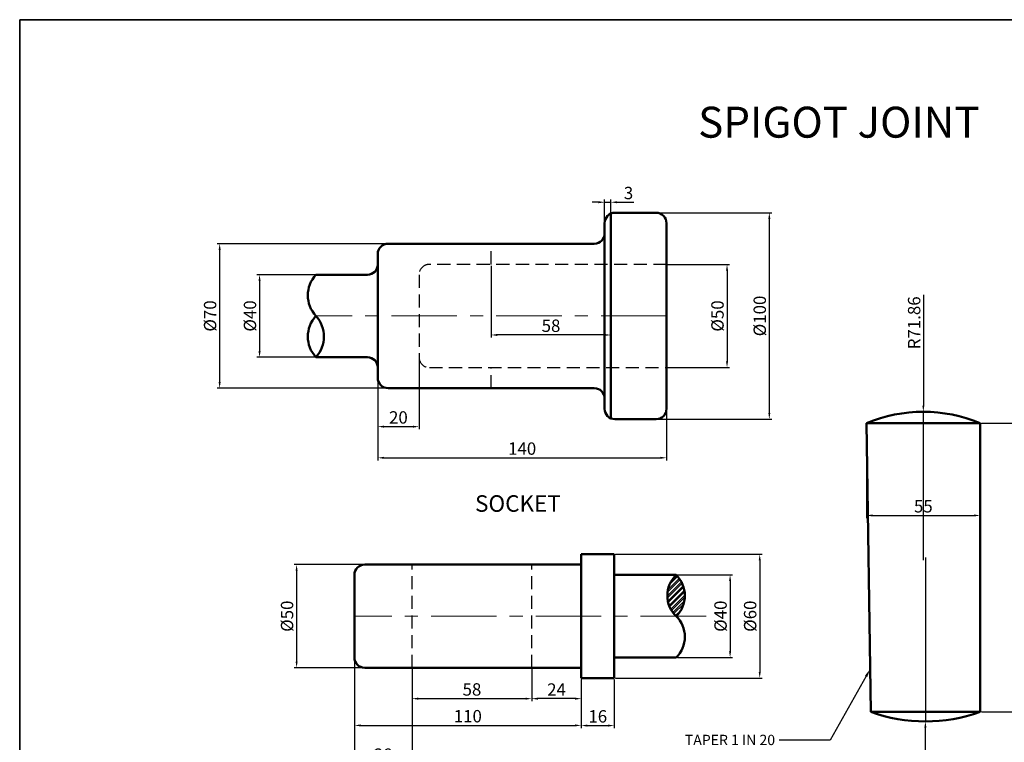
# Model space of a CAD drawing. Units: millimetres. Extents: x 641 to 1388, y -43 to 643.
# Tile 2 of 3: x 641 to 1119, y 293 to 643. Entities that reach past the tile are written whole.
import ezdxf
from ezdxf import colors
from ezdxf.entities.mleader import LeaderData, LeaderLine
from ezdxf.math import Vec2, Vec3

# ---------------------------------------------------------------- set-up
doc = ezdxf.new("R2010")
doc.units = ezdxf.units.MM
doc.linetypes.add('CENTER', pattern=[50.8, 31.75, -6.35, 6.35, -6.35])
doc.linetypes.add('HIDDEN', pattern=[9.525, 6.35, -3.175])
for name, color, linetype, lineweight in [('M-CNTR', 1, 'CENTER', 18), ('M-DIMS', 2, 'Continuous', 25), ('M-HATC', 8, 'Continuous', 18), ('M-HIDN', 4, 'HIDDEN', 25), ('M-OUTL', 7, 'Continuous', 50), ('M-TEXT', 3, 'Continuous', 25), ('M-TTLB', 7, 'Continuous', 35)]:
    doc.layers.add(name, color=color, linetype=linetype, lineweight=lineweight)
doc.styles.get("Standard").update_dxf_attribs({"font": 'arial.ttf'})
doc.dimstyles.new('ISO-25', dxfattribs={"dimtxt": 6, "dimasz": 3, "dimexe": 1.25, "dimexo": 0.625, "dimtad": 1, "dimdec": 0, "dimtxsty": 'Standard', "dimcen": 2.5, "dimadec": 0, "dimazin": 0, "dimtfac": 1, "dimtdec": 0, "dimtmove": 0, "dimatfit": 3, "dimfxl": 1, "dimarcsym": 0})

# ---------------------------------------------------------------- blocks, each defined once
blk = doc.blocks.new('*D1')
at = {"layer": 'Defpoints', "color": 0, "transparency": 16777216}
for p in [(949.99, 549.27), (949.99, 449.27), (1004.85, 449.27)]:
    blk.add_point(p, dxfattribs=at)
at = {"layer": 'M-DIMS', "color": 0, "lineweight": -2, "transparency": 16777216}
for p, q in [((950.61, 549.27), (1006.1, 549.27)), ((1004.85, 546.27), (1004.85, 452.27)), ((950.61, 449.27), (1006.1, 449.27))]:
    blk.add_line(p, q, dxfattribs=at)
at = {"layer": 'M-DIMS', "color": 0, "transparency": 16777216}
for points in [[(1004.35, 546.27), (1005.35, 546.27), (1004.85, 549.27)], [(1004.35, 452.27), (1005.35, 452.27), (1004.85, 449.27)]]:
    blk.add_solid(points, dxfattribs=at)
at = {"layer": 'M-DIMS', "color": 0, "transparency": 16777216, "insert": (1000.99, 499.27), "char_height": 6, "attachment_point": 5, "rotation": 90}
blk.add_mtext('%%C100', dxfattribs=at)
blk = doc.blocks.new('*D2')
at = {"layer": 'Defpoints', "color": 0, "transparency": 16777216}
for p in [(954.99, 524.27), (954.99, 474.27), (984.34, 474.27)]:
    blk.add_point(p, dxfattribs=at)
at = {"layer": 'M-DIMS', "color": 0, "lineweight": -2, "transparency": 16777216}
for p, q in [((955.61, 524.27), (985.59, 524.27)), ((984.34, 521.27), (984.34, 477.27)), ((955.61, 474.27), (985.59, 474.27))]:
    blk.add_line(p, q, dxfattribs=at)
at = {"layer": 'M-DIMS', "color": 0, "transparency": 16777216}
for points in [[(983.84, 521.27), (984.84, 521.27), (984.34, 524.27)], [(983.84, 477.27), (984.84, 477.27), (984.34, 474.27)]]:
    blk.add_solid(points, dxfattribs=at)
at = {"layer": 'M-DIMS', "color": 0, "transparency": 16777216, "insert": (980.49, 499.27), "char_height": 6, "attachment_point": 5, "rotation": 90}
blk.add_mtext('%%C50', dxfattribs=at)
blk = doc.blocks.new('*D3')
at = {"layer": 'Defpoints', "color": 0, "transparency": 16777216}
for p in [(819.99, 534.27), (738.31, 464.27), (819.99, 464.27)]:
    blk.add_point(p, dxfattribs=at)
at = {"layer": 'M-DIMS', "color": 0, "lineweight": -2, "transparency": 16777216}
for p, q in [((819.36, 534.27), (737.06, 534.27)), ((738.31, 531.27), (738.31, 467.27)), ((819.36, 464.27), (737.06, 464.27))]:
    blk.add_line(p, q, dxfattribs=at)
at = {"layer": 'M-DIMS', "color": 0, "transparency": 16777216}
for points in [[(737.81, 531.27), (738.81, 531.27), (738.31, 534.27)], [(737.81, 467.27), (738.81, 467.27), (738.31, 464.27)]]:
    blk.add_solid(points, dxfattribs=at)
at = {"layer": 'M-DIMS', "color": 0, "transparency": 16777216, "insert": (734.46, 499.27), "char_height": 6, "attachment_point": 5, "rotation": 90}
blk.add_mtext('%%C70', dxfattribs=at)
blk = doc.blocks.new('*D4')
at = {"layer": 'Defpoints', "color": 0, "transparency": 16777216}
for p in [(790.87, 519.27), (757.66, 479.27), (790.87, 479.27)]:
    blk.add_point(p, dxfattribs=at)
at = {"layer": 'M-DIMS', "color": 0, "lineweight": -2, "transparency": 16777216}
for p, q in [((790.25, 519.27), (756.41, 519.27)), ((757.66, 516.27), (757.66, 482.27)), ((790.25, 479.27), (756.41, 479.27))]:
    blk.add_line(p, q, dxfattribs=at)
at = {"layer": 'M-DIMS', "color": 0, "transparency": 16777216}
for points in [[(757.16, 516.27), (758.16, 516.27), (757.66, 519.27)], [(757.16, 482.27), (758.16, 482.27), (757.66, 479.27)]]:
    blk.add_solid(points, dxfattribs=at)
at = {"layer": 'M-DIMS', "color": 0, "transparency": 16777216, "insert": (753.8, 499.27), "char_height": 6, "attachment_point": 5, "rotation": 90}
blk.add_mtext('%%C40', dxfattribs=at)
blk = doc.blocks.new('*D5')
at = {"layer": 'Defpoints', "color": 0, "transparency": 16777216}
for p in [(927.99, 554.39), (924.99, 541.77), (927.99, 541.77)]:
    blk.add_point(p, dxfattribs=at)
at = {"layer": 'M-DIMS', "color": 0, "lineweight": -2, "transparency": 16777216}
for p, q in [((921.99, 554.39), (918.99, 554.39)), ((924.99, 542.4), (924.99, 555.64)), ((924.99, 554.39), (927.99, 554.39)), ((927.99, 542.4), (927.99, 555.64)), ((930.99, 554.39), (939.17, 554.39))]:
    blk.add_line(p, q, dxfattribs=at)
at = {"layer": 'M-DIMS', "color": 0, "transparency": 16777216}
for points in [[(921.99, 554.89), (921.99, 553.89), (924.99, 554.39)], [(930.99, 554.89), (930.99, 553.89), (927.99, 554.39)]]:
    blk.add_solid(points, dxfattribs=at)
at = {"layer": 'M-DIMS', "color": 0, "transparency": 16777216, "insert": (936.58, 558.08), "char_height": 6, "attachment_point": 5}
blk.add_mtext('3', dxfattribs=at)
blk = doc.blocks.new('*D6')
at = {"layer": 'Defpoints', "color": 0, "transparency": 16777216}
for p in [(869.99, 524.27), (927.99, 499.27), (869.99, 490.07)]:
    blk.add_point(p, dxfattribs=at)
at = {"layer": 'M-DIMS', "color": 0, "lineweight": -2, "transparency": 16777216}
for p, q in [((869.99, 523.65), (869.99, 488.82)), ((927.99, 498.65), (927.99, 488.82)), ((924.99, 490.07), (872.99, 490.07))]:
    blk.add_line(p, q, dxfattribs=at)
at = {"layer": 'M-DIMS', "color": 0, "transparency": 16777216}
for points in [[(872.99, 490.57), (872.99, 489.57), (869.99, 490.07)], [(924.99, 490.57), (924.99, 489.57), (927.99, 490.07)]]:
    blk.add_solid(points, dxfattribs=at)
at = {"layer": 'M-DIMS', "color": 0, "transparency": 16777216, "insert": (898.99, 493.76), "char_height": 6, "attachment_point": 5}
blk.add_mtext('58', dxfattribs=at)
blk = doc.blocks.new('*D7')
at = {"layer": 'Defpoints', "color": 0, "transparency": 16777216}
for p in [(814.99, 469.27), (954.99, 469.27), (954.99, 430.55)]:
    blk.add_point(p, dxfattribs=at)
at = {"layer": 'M-DIMS', "color": 0, "lineweight": -2, "transparency": 16777216}
for p, q in [((814.99, 468.65), (814.99, 429.3)), ((954.99, 468.65), (954.99, 429.3)), ((817.99, 430.55), (951.99, 430.55))]:
    blk.add_line(p, q, dxfattribs=at)
at = {"layer": 'M-DIMS', "color": 0, "transparency": 16777216}
for points in [[(817.99, 431.05), (817.99, 430.05), (814.99, 430.55)], [(951.99, 431.05), (951.99, 430.05), (954.99, 430.55)]]:
    blk.add_solid(points, dxfattribs=at)
at = {"layer": 'M-DIMS', "color": 0, "transparency": 16777216, "insert": (884.99, 434.23), "char_height": 6, "attachment_point": 5}
blk.add_mtext('140', dxfattribs=at)
blk = doc.blocks.new('*D8')
at = {"layer": 'Defpoints', "color": 0, "transparency": 16777216}
for p in [(814.99, 496.77), (834.99, 479.27), (834.99, 445.64)]:
    blk.add_point(p, dxfattribs=at)
at = {"layer": 'M-DIMS', "color": 0, "lineweight": -2, "transparency": 16777216}
for p, q in [((814.99, 496.15), (814.99, 444.39)), ((834.99, 478.65), (834.99, 444.39)), ((817.99, 445.64), (831.99, 445.64))]:
    blk.add_line(p, q, dxfattribs=at)
at = {"layer": 'M-DIMS', "color": 0, "transparency": 16777216}
for points in [[(817.99, 446.14), (817.99, 445.14), (814.99, 445.64)], [(831.99, 446.14), (831.99, 445.14), (834.99, 445.64)]]:
    blk.add_solid(points, dxfattribs=at)
at = {"layer": 'M-DIMS', "color": 0, "transparency": 16777216, "insert": (824.99, 449.33), "char_height": 6, "attachment_point": 5}
blk.add_mtext('20', dxfattribs=at)
blk = doc.blocks.new('*D9')
at = {"layer": 'Defpoints', "color": 0, "transparency": 16777216}
for p in [(1107.03, 447.38), (1107.03, 307.38), (1140.01, 307.38)]:
    blk.add_point(p, dxfattribs=at)
at = {"layer": 'M-DIMS', "color": 0, "lineweight": -2, "transparency": 16777216}
for p, q in [((1107.65, 447.38), (1141.26, 447.38)), ((1140.01, 444.38), (1140.01, 310.38)), ((1107.65, 307.38), (1141.26, 307.38))]:
    blk.add_line(p, q, dxfattribs=at)
at = {"layer": 'M-DIMS', "color": 0, "transparency": 16777216}
for points in [[(1139.51, 444.38), (1140.51, 444.38), (1140.01, 447.38)], [(1139.51, 310.38), (1140.51, 310.38), (1140.01, 307.38)]]:
    blk.add_solid(points, dxfattribs=at)
at = {"layer": 'M-DIMS', "color": 0, "transparency": 16777216, "insert": (1136.32, 377.38), "char_height": 6, "attachment_point": 5, "rotation": 90}
blk.add_mtext('140', dxfattribs=at)
blk = doc.blocks.new('*D10')
at = {"layer": 'Defpoints', "color": 0, "transparency": 16777216}
for p in [(1052.03, 447.38), (1107.03, 447.38), (1107.03, 402.6)]:
    blk.add_point(p, dxfattribs=at)
at = {"layer": 'M-DIMS', "color": 0, "lineweight": -2, "transparency": 16777216}
for p, q in [((1052.03, 446.75), (1052.03, 401.35)), ((1107.03, 446.75), (1107.03, 401.35)), ((1055.03, 402.6), (1104.03, 402.6))]:
    blk.add_line(p, q, dxfattribs=at)
at = {"layer": 'M-DIMS', "color": 0, "transparency": 16777216}
for points in [[(1055.03, 403.1), (1055.03, 402.1), (1052.03, 402.6)], [(1104.03, 403.1), (1104.03, 402.1), (1107.03, 402.6)]]:
    blk.add_solid(points, dxfattribs=at)
at = {"layer": 'M-DIMS', "color": 0, "transparency": 16777216, "insert": (1079.53, 406.28), "char_height": 6, "attachment_point": 5}
blk.add_mtext('55', dxfattribs=at)
blk = doc.blocks.new('*D11')
at = {"layer": 'Defpoints', "color": 0, "transparency": 16777216}
for p in [(817.55, 378.79), (775.63, 328.79), (817.55, 328.79)]:
    blk.add_point(p, dxfattribs=at)
at = {"layer": 'M-DIMS', "color": 0, "lineweight": -2, "transparency": 16777216}
for p, q in [((816.92, 378.79), (774.38, 378.79)), ((775.63, 375.79), (775.63, 331.79)), ((816.92, 328.79), (774.38, 328.79))]:
    blk.add_line(p, q, dxfattribs=at)
at = {"layer": 'M-DIMS', "color": 0, "transparency": 16777216}
for points in [[(775.13, 375.79), (776.13, 375.79), (775.63, 378.79)], [(775.13, 331.79), (776.13, 331.79), (775.63, 328.79)]]:
    blk.add_solid(points, dxfattribs=at)
at = {"layer": 'M-DIMS', "color": 0, "transparency": 16777216, "insert": (771.77, 353.79), "char_height": 6, "attachment_point": 5, "rotation": 90}
blk.add_mtext('%%C50', dxfattribs=at)
blk = doc.blocks.new('*D12')
at = {"layer": 'Defpoints', "color": 0, "transparency": 16777216}
for p in [(831.65, 328.79), (889.65, 328.79), (889.65, 313.83)]:
    blk.add_point(p, dxfattribs=at)
at = {"layer": 'M-DIMS', "color": 0, "lineweight": -2, "transparency": 16777216}
for p, q in [((831.65, 328.16), (831.65, 312.58)), ((889.65, 328.16), (889.65, 312.58)), ((834.65, 313.83), (886.65, 313.83))]:
    blk.add_line(p, q, dxfattribs=at)
at = {"layer": 'M-DIMS', "color": 0, "transparency": 16777216}
for points in [[(834.65, 314.33), (834.65, 313.33), (831.65, 313.83)], [(886.65, 314.33), (886.65, 313.33), (889.65, 313.83)]]:
    blk.add_solid(points, dxfattribs=at)
at = {"layer": 'M-DIMS', "color": 0, "transparency": 16777216, "insert": (860.65, 317.52), "char_height": 6, "attachment_point": 5}
blk.add_mtext('58', dxfattribs=at)
blk = doc.blocks.new('*D13')
at = {"layer": 'Defpoints', "color": 0, "transparency": 16777216}
for p in [(889.65, 323.79), (913.65, 323.79), (889.65, 313.83)]:
    blk.add_point(p, dxfattribs=at)
at = {"layer": 'M-DIMS', "color": 0, "lineweight": -2, "transparency": 16777216}
for p, q in [((889.65, 323.16), (889.65, 312.58)), ((913.65, 323.16), (913.65, 312.58)), ((910.65, 313.83), (892.65, 313.83))]:
    blk.add_line(p, q, dxfattribs=at)
at = {"layer": 'M-DIMS', "color": 0, "transparency": 16777216}
for points in [[(892.65, 314.33), (892.65, 313.33), (889.65, 313.83)], [(910.65, 314.33), (910.65, 313.33), (913.65, 313.83)]]:
    blk.add_solid(points, dxfattribs=at)
at = {"layer": 'M-DIMS', "color": 0, "transparency": 16777216, "insert": (901.65, 317.47), "char_height": 6, "attachment_point": 5}
blk.add_mtext('24', dxfattribs=at)
blk = doc.blocks.new('*D14')
at = {"layer": 'Defpoints', "color": 0, "transparency": 16777216}
for p in [(913.65, 323.79), (929.65, 323.79), (929.65, 300.79)]:
    blk.add_point(p, dxfattribs=at)
at = {"layer": 'M-DIMS', "color": 0, "lineweight": -2, "transparency": 16777216}
for p, q in [((913.65, 323.16), (913.65, 299.54)), ((929.65, 323.16), (929.65, 299.54)), ((916.65, 300.79), (926.65, 300.79))]:
    blk.add_line(p, q, dxfattribs=at)
at = {"layer": 'M-DIMS', "color": 0, "transparency": 16777216}
for points in [[(916.65, 301.29), (916.65, 300.29), (913.65, 300.79)], [(926.65, 301.29), (926.65, 300.29), (929.65, 300.79)]]:
    blk.add_solid(points, dxfattribs=at)
at = {"layer": 'M-DIMS', "color": 0, "transparency": 16777216, "insert": (921.65, 304.48), "char_height": 6, "attachment_point": 5}
blk.add_mtext('16', dxfattribs=at)
blk = doc.blocks.new('*D15')
at = {"layer": 'Defpoints', "color": 0, "transparency": 16777216}
for p in [(803.65, 340.69), (913.65, 310.42), (913.65, 300.87)]:
    blk.add_point(p, dxfattribs=at)
at = {"layer": 'M-DIMS', "color": 0, "lineweight": -2, "transparency": 16777216}
for p, q in [((803.65, 340.06), (803.65, 299.62)), ((913.65, 309.8), (913.65, 299.62)), ((806.65, 300.87), (910.65, 300.87))]:
    blk.add_line(p, q, dxfattribs=at)
at = {"layer": 'M-DIMS', "color": 0, "transparency": 16777216}
for points in [[(806.65, 301.37), (806.65, 300.37), (803.65, 300.87)], [(910.65, 301.37), (910.65, 300.37), (913.65, 300.87)]]:
    blk.add_solid(points, dxfattribs=at)
at = {"layer": 'M-DIMS', "color": 0, "transparency": 16777216, "insert": (858.65, 304.56), "char_height": 6, "attachment_point": 5}
blk.add_mtext('110', dxfattribs=at)
blk = doc.blocks.new('*D16')
at = {"layer": 'Defpoints', "color": 0, "transparency": 16777216}
for p in [(959.65, 373.79), (959.65, 333.79), (985.82, 333.79)]:
    blk.add_point(p, dxfattribs=at)
at = {"layer": 'M-DIMS', "color": 0, "lineweight": -2, "transparency": 16777216}
for p, q in [((960.27, 373.79), (987.07, 373.79)), ((985.82, 370.79), (985.82, 336.79)), ((960.27, 333.79), (987.07, 333.79))]:
    blk.add_line(p, q, dxfattribs=at)
at = {"layer": 'M-DIMS', "color": 0, "transparency": 16777216}
for points in [[(985.32, 370.79), (986.32, 370.79), (985.82, 373.79)], [(985.32, 336.79), (986.32, 336.79), (985.82, 333.79)]]:
    blk.add_solid(points, dxfattribs=at)
at = {"layer": 'M-DIMS', "color": 0, "transparency": 16777216, "insert": (981.97, 353.79), "char_height": 6, "attachment_point": 5, "rotation": 90}
blk.add_mtext('%%C40', dxfattribs=at)
blk = doc.blocks.new('*D17')
at = {"layer": 'Defpoints', "color": 0, "transparency": 16777216}
for p in [(929.65, 383.79), (929.65, 323.79), (1000.19, 323.79)]:
    blk.add_point(p, dxfattribs=at)
at = {"layer": 'M-DIMS', "color": 0, "lineweight": -2, "transparency": 16777216}
for p, q in [((930.27, 383.79), (1001.44, 383.79)), ((1000.19, 380.79), (1000.19, 326.79)), ((930.27, 323.79), (1001.44, 323.79))]:
    blk.add_line(p, q, dxfattribs=at)
at = {"layer": 'M-DIMS', "color": 0, "transparency": 16777216}
for points in [[(999.69, 380.79), (1000.69, 380.79), (1000.19, 383.79)], [(999.69, 326.79), (1000.69, 326.79), (1000.19, 323.79)]]:
    blk.add_solid(points, dxfattribs=at)
at = {"layer": 'M-DIMS', "color": 0, "transparency": 16777216, "insert": (996.33, 353.79), "char_height": 6, "attachment_point": 5, "rotation": 90}
blk.add_mtext('%%C60', dxfattribs=at)
blk = doc.blocks.new('COTTER')
for p, q in [((0, 144.55), (55, 144.55)), ((2, 4.55), (0, 144.55)), ((55, 144.55), (55, 4.55)), ((55, 4.55), (2, 4.55)), ((2, 4.55), (4, 4.55)), ((2, 4.55), (4, 4.55))]:
    blk.add_line(p, q)
for centre, radius, start, end in [((27.5, 78.16), 71.86, 67.5, 112.5), ((28.5, 79.43), 79.43, 250.5117, 289.4883)]:
    blk.add_arc(centre, radius, start, end)
blk = doc.blocks.new('*D32')
at = {"layer": 'Defpoints', "color": 0, "transparency": 16777216}
for p in [(803.65, 333.79), (831.65, 328.79), (831.65, 282.23)]:
    blk.add_point(p, dxfattribs=at)
at = {"layer": 'M-DIMS', "color": 0, "lineweight": -2, "transparency": 16777216}
for p, q in [((803.65, 333.16), (803.65, 280.98)), ((831.65, 328.16), (831.65, 280.98)), ((806.65, 282.23), (828.65, 282.23))]:
    blk.add_line(p, q, dxfattribs=at)
at = {"layer": 'M-DIMS', "color": 0, "transparency": 16777216}
for points in [[(806.65, 282.73), (806.65, 281.73), (803.65, 282.23)], [(828.65, 282.73), (828.65, 281.73), (831.65, 282.23)]]:
    blk.add_solid(points, dxfattribs=at)
at = {"layer": 'M-DIMS', "color": 0, "transparency": 16777216, "insert": (817.65, 285.91), "char_height": 6, "attachment_point": 5}
blk.add_mtext('28', dxfattribs=at)
blk = doc.blocks.new('*D33')
at = {"layer": 'Defpoints', "color": 0, "transparency": 16777216}
for p in [(1080.53, 382.26), (1080.53, 302.83)]:
    blk.add_point(p, dxfattribs=at)
at = {"layer": 'M-DIMS', "color": 0, "lineweight": -2, "transparency": 16777216}
for p, q in [((1080.53, 382.26), (1080.53, 302.83)), ((1080.53, 241.55), (1080.53, 299.83))]:
    blk.add_line(p, q, dxfattribs=at)
at = {"layer": 'M-DIMS', "color": 0, "transparency": 16777216}
blk.add_solid([(1081.03, 299.83), (1080.03, 299.83), (1080.53, 302.83)], dxfattribs=at)
at = {"layer": 'M-DIMS', "color": 0, "transparency": 16777216, "insert": (1084.22, 255.17), "char_height": 6, "attachment_point": 5, "rotation": 270.0002}
blk.add_mtext('R79.43', dxfattribs=at)
blk = doc.blocks.new('*D34')
at = {"layer": 'Defpoints', "color": 0, "transparency": 16777216}
for p in [(1079.53, 452.85), (1079.53, 380.99)]:
    blk.add_point(p, dxfattribs=at)
at = {"layer": 'M-DIMS', "color": 0, "lineweight": -2, "transparency": 16777216}
for p, q in [((1079.53, 509.58), (1079.53, 455.85)), ((1079.53, 380.99), (1079.53, 452.85))]:
    blk.add_line(p, q, dxfattribs=at)
at = {"layer": 'M-DIMS', "color": 0, "transparency": 16777216}
blk.add_solid([(1079.03, 455.85), (1080.03, 455.85), (1079.53, 452.85)], dxfattribs=at)
at = {"layer": 'M-DIMS', "color": 0, "transparency": 16777216, "insert": (1075.84, 495.96), "char_height": 6, "attachment_point": 5, "rotation": 89.9997}
blk.add_mtext('R71.86', dxfattribs=at)

msp = doc.modelspace()

# ---------------------------------------------------------------- hatches: boundary and pattern name
at = {"layer": 'M-HATC'}
h = msp.add_hatch(dxfattribs=at)
h.set_pattern_fill('ANSI32', color=256, scale=0.2)
h.set_pattern_definition([(45, (719.972, 680.44), (-1.347038, 1.347038), []), (45, (720.87, 680.44), (-1.347038, 1.347038), [])])
h.paths.add_polyline_path([(959.65, 353.786, 0.4249028), (959.65, 373.786, 0.4249028)])

# ---------------------------------------------------------------- linework, layer by layer
at = {"layer": 'M-CNTR'}
for p, q in [((954.988, 499.275), (784.988, 499.275)), ((974.145, 353.786), (803.65, 353.786))]:
    msp.add_line(p, q, dxfattribs=at)
at = {"layer": 'M-HIDN'}
for p, q in [((869.988, 524.275), (869.988, 534.275)), ((869.988, 464.275), (869.988, 474.275)), ((831.65, 328.786), (831.65, 378.786)), ((889.65, 328.786), (889.65, 378.786))]:
    msp.add_line(p, q, dxfattribs=at)
msp.add_lwpolyline([(954.988, 524.275), (839.988, 524.275, 0.4142136), (834.988, 519.275), (834.988, 479.275, 0.4142136), (839.988, 474.275), (954.988, 474.275)], format="xyb", dxfattribs=at)
at = {"layer": 'M-OUTL'}
for p, q in [((929.988, 549.275), (949.988, 549.275)), ((927.988, 449.692), (927.988, 548.857)), ((924.988, 539.275), (924.988, 544.275)), ((954.988, 544.275), (954.988, 454.275)), ((924.988, 459.275), (924.988, 539.275)), ((819.988, 534.275), (919.988, 534.275)), ((814.988, 524.275), (814.988, 529.275)), ((814.988, 469.275), (814.988, 524.275)), ((809.988, 519.275), (784.988, 519.275)), ((784.988, 479.275), (809.988, 479.275)), ((819.988, 464.275), (919.988, 464.275)), ((924.988, 454.275), (924.988, 459.275)), ((949.988, 449.275), (929.988, 449.275)), ((929.65, 383.786), (913.65, 383.786)), ((913.65, 383.786), (913.65, 323.786)), ((929.65, 323.786), (929.65, 383.786)), ((808.65, 378.786), (913.65, 378.786)), ((803.65, 333.786), (803.65, 373.786)), ((929.65, 373.786), (959.65, 373.786)), ((959.65, 333.786), (929.65, 333.786)), ((808.65, 328.786), (913.65, 328.786)), ((913.65, 323.786), (929.65, 323.786))]:
    msp.add_line(p, q, dxfattribs=at)
for centre, radius, start, end in [((929.988, 544.275), 5, 90, 180), ((949.988, 544.275), 5, 0, 90), ((919.988, 539.275), 5, 270, 0), ((819.988, 529.275), 5, 90, 180), ((809.988, 524.275), 5, 270, 0), ((795.81, 509.275), 14.735, 137.26103, 222.73897), ((795.81, 489.275), 14.735, 137.26103, 222.73897), ((774.166, 489.275), 14.735, 317.26103, 42.73897), ((809.988, 474.275), 5, 0, 90), ((819.988, 469.275), 5, 180, 270), ((919.988, 459.275), 5, 0, 90), ((929.988, 454.275), 5, 180, 270), ((949.988, 454.275), 5, 270, 0), ((808.65, 373.786), 5, 90, 180), ((969.293, 363.786), 13.892, 133.95845, 226.04155), ((950.007, 363.786), 13.892, 313.95845, 46.04155), ((950.007, 343.786), 13.892, 313.95845, 46.04155), ((808.65, 333.786), 5, 180, 270)]:
    msp.add_arc(centre, radius, start, end, dxfattribs=at)
at = {"layer": 'M-TTLB'}
msp.add_lwpolyline([(641.348, 642.837), (1388.388, 642.837), (1388.388, -42.647), (641.348, -42.647)], close=True, dxfattribs=at)

# ---------------------------------------------------------------- block references
at = {"layer": 'M-OUTL'}
msp.add_blockref('COTTER', (1052.03, 302.826), dxfattribs=at)

# ---------------------------------------------------------------- texts
at = {"layer": 'M-TEXT', "attachment_point": 1}
for s, width, insert, char_height in [('SPIGOT JOINT', 190.57708, (970.334, 600.677), 15), ('\\pxqc;SOCKET', 125.14088, (820.372, 412.396), 8)]:
    msp.add_mtext_dynamic_manual_height_columns(s, width=width, gutter_width=12.5, heights=[0], dxfattribs=dict(at, insert=insert, char_height=char_height))

# ---------------------------------------------------------------- dimensions: what is measured, and where the dimension line sits
at = {"layer": 'M-DIMS'}
for base, p1, p2, override, picture, middle in [((927.988, 554.388), (924.988, 541.775), (927.988, 541.775), {"dimclrd": 0, "dimclre": 0, "dimclrt": 0}, '*D5', (936.578, 558.079)), ((869.988, 490.067), (927.988, 499.275), (869.988, 524.275), {"dimclrd": 0, "dimclre": 0, "dimclrt": 0}, '*D6', (898.988, 493.755)), ((834.988, 445.644), (814.988, 496.775), (834.988, 479.275), {"dimclrd": 0, "dimclre": 0, "dimclrt": 0}, '*D8', (824.988, 449.333)), ((954.988, 430.545), (814.988, 469.275), (954.988, 469.275), {"dimclrd": 0, "dimclre": 0, "dimclrt": 0}, '*D7', (884.988, 434.234)), ((1107.03, 402.604), (1052.03, 447.376), (1107.03, 447.376), {"dimclrd": 0, "dimclre": 0, "dimclrt": 0}, '*D10', (1079.53, 406.28)), ((913.65, 300.874), (803.65, 340.685), (913.65, 310.422), {"dimclrd": 0, "dimclre": 0, "dimclrt": 0}, '*D15', (858.65, 304.562)), ((831.65, 282.226), (803.65, 333.786), (831.65, 328.786), {"dimdec": 0, "dimlfac": 1, "dimrnd": 0, "dimzin": 0, "dimdsep": 46, "dimlunit": 2}, '*D32', (817.65, 285.914)), ((889.65, 313.831), (831.65, 328.786), (889.65, 328.786), {"dimclrd": 0, "dimclre": 0, "dimclrt": 0}, '*D12', (860.65, 317.52)), ((889.65, 313.831), (913.65, 323.786), (889.65, 323.786), {"dimclrd": 0, "dimclre": 0, "dimclrt": 0}, '*D13', (901.65, 317.469))]:
    dim = msp.add_linear_dim(base=base, p1=p1, p2=p2, dimstyle='ISO-25', override=override, dxfattribs=at)
    dim.commit()
    dim.dimension.update_dxf_attribs({"geometry": picture, "text_midpoint": middle})
for base, p1, p2, picture, middle in [((1004.85, 449.275), (949.988, 549.275), (949.988, 449.275), '*D1', (1000.994, 499.275)), ((738.312, 464.275), (819.988, 534.275), (819.988, 464.275), '*D3', (734.455, 499.275)), ((984.343, 474.275), (954.988, 524.275), (954.988, 474.275), '*D2', (980.486, 499.275)), ((757.655, 479.275), (790.871, 519.275), (790.871, 479.275), '*D4', (753.799, 499.275)), ((1000.186, 323.786), (929.65, 383.786), (929.65, 323.786), '*D17', (996.33, 353.786)), ((775.625, 328.786), (817.545, 378.786), (817.545, 328.786), '*D11', (771.769, 353.786)), ((985.823, 333.786), (959.65, 373.786), (959.65, 333.786), '*D16', (981.967, 353.786))]:
    dim = msp.add_linear_dim(base=base, p1=p1, p2=p2, angle=90, text='%%C<>', dimstyle='ISO-25', override={"dimclrd": 0, "dimclre": 0, "dimclrt": 0}, dxfattribs=at)
    dim.commit()
    dim.dimension.update_dxf_attribs({"geometry": picture, "text_midpoint": middle})
for center, mpoint, picture, middle in [((1079.53, 380.986), (1079.53, 452.846), '*D34', (1079.53, 495.963)), ((1080.53, 382.259), (1080.53, 302.826), '*D33', (1080.53, 255.166))]:
    dim = msp.add_radius_dim(center=center, mpoint=mpoint, dimstyle='ISO-25', override={"dimdec": 2, "dimlfac": 1, "dimrnd": 0, "dimzin": 0, "dimdsep": 46, "dimlunit": 2}, dxfattribs=at)
    dim.commit()
    dim.dimension.update_dxf_attribs({"geometry": picture, "text_midpoint": middle, "dimtype": 164})
dim = msp.add_linear_dim(base=(1140.008, 307.376), p1=(1107.03, 447.376), p2=(1107.03, 307.376), angle=90, dimstyle='ISO-25', override={"dimclrd": 0, "dimclre": 0, "dimclrt": 0}, dxfattribs=at)
dim.commit()
dim.dimension.update_dxf_attribs({"geometry": '*D9', "text_midpoint": (1136.319, 377.376)})
dim = msp.add_linear_dim(base=(929.65, 300.793), p1=(913.65, 323.786), p2=(929.65, 323.786), dimstyle='ISO-25', override={"dimclrd": 0, "dimclre": 0, "dimclrt": 0}, dxfattribs=at)
dim.commit()
dim.dimension.update_dxf_attribs({"geometry": '*D14', "text_midpoint": (921.65, 300.793), "dimtype": 160})

# ---------------------------------------------------------------- leaders
at = {"layer": 'M-TEXT'}
ml = msp.add_multileader_mtext('Standard', dxfattribs=at)
ml.set_content('TAPER 1 IN 20 \\P\\pxqc;THICKNESS 14', color=256)
ml.set_leader_properties()
ml.build(insert=Vec2(0, 0))
ctx = ml.context
ctx.base_point, ctx.char_height, ctx.plane_origin = Vec3(956.457, 293.786), 5, Vec3(1053.733, 328.138)
ctx.text_align_type = 2
notes = []
notes.append((ctx, [(0, (1, 1, 0), (1034.33, 293.786), (-1, 0), 24.688, [(0, [(1053.733, 328.138)], 0, [])])]))
ctx.mtext.insert, ctx.mtext.alignment, ctx.mtext.flow_direction = Vec3(1007.642, 296.329), 3, 5
for ctx, leaders in notes:
    for number, flags, end, landing, length, lines in leaders:
        leader = LeaderData()
        leader.index, (leader.has_last_leader_line, leader.has_dogleg_vector, leader.attachment_direction) = number, flags
        leader.last_leader_point, leader.dogleg_vector, leader.dogleg_length = Vec3(end), Vec3(landing), length
        for number, points, colour, breaks in lines:
            line = LeaderLine()
            line.index, line.vertices, line.color, line.breaks = number, Vec3.list(points), colors.encode_raw_color(colour), breaks
            leader.lines.append(line)
        ctx.leaders.append(leader)

doc.saveas('drawing.dxf')
